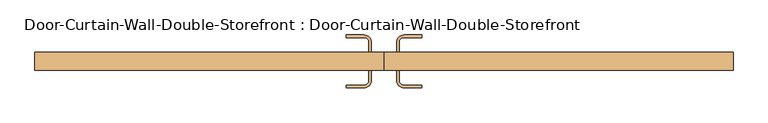
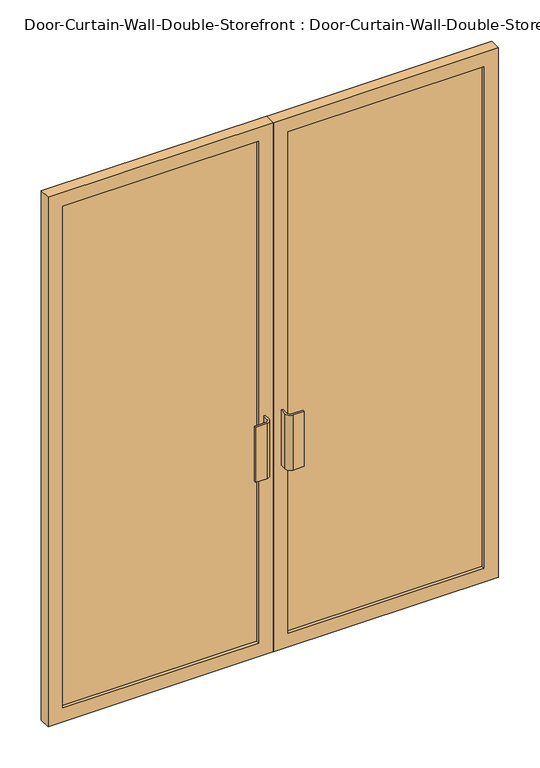
"""IFC4 building model written with IfcOpenShell, lengths in millimetres: door geometry, Door-Curtain-Wall-Double-Storefront : Door-Curtain-Wall-Double-Storefront."""

from ifc_helpers import new_model, si_unit, point, frame, frame_2d, origin, place, context, project, spatial, polyline, circle_curve, trimmed, segment, composite_curve, outline, extrude, source, transform, mapped, element, save


def door_curtain_wall_double_storefront_door_curtain_wall_double_c727979e(model_context):
    return source(origin(), model_context, "Body", "SweptSolid", [
        extrude(outline(polyline([(2190.75, 0.7668501), (0.0, 0.7668501), (0.0, 882.65), (2190.75, 882.65), (2190.75, 0.7668501)]), holes=[polyline([(2133.6, 57.9168501), (2133.6, 825.5), (57.15, 825.5), (57.15, 57.9168501), (2133.6, 57.9168501)])]), frame((0.0, 12.7, 0.0), z_axis=(0.0, 1.0, 0.0), x_axis=(0.0, 0.0, 1.0)), (0.0, 0.0, 1.0), 44.45),
        extrude(outline(polyline([(2190.75, -0.8206499), (2190.75, -882.65), (0.0, -882.65), (0.0, -0.8206499), (2190.75, -0.8206499)]), holes=[polyline([(2133.6, -825.5), (2133.6, -57.9706499), (57.15, -57.9706499), (57.15, -825.5), (2133.6, -825.5)])]), frame((0.0, 12.7, 0.0), z_axis=(0.0, 1.0, 0.0), x_axis=(0.0, 0.0, 1.0)), (0.0, 0.0, 1.0), 44.45),
        extrude(outline(polyline([(825.5, 25.4), (57.9168501, 25.4), (57.9168501, 44.45), (825.5, 44.45), (825.5, 25.4)])), frame((0.0, 0.0, 57.15), z_axis=(0.0, 0.0, 1.0), x_axis=(1.0, 0.0, 0.0)), (0.0, 0.0, 1.0), 2076.45),
        extrude(outline(polyline([(-57.9706499, 25.4), (-825.5, 25.4), (-825.5, 44.45), (-57.9706499, 44.45), (-57.9706499, 25.4)])), frame((0.0, 0.0, 57.15), z_axis=(0.0, 0.0, 1.0), x_axis=(1.0, 0.0, 0.0)), (0.0, 0.0, 1.0), 2076.45),
        extrude(outline(composite_curve([segment(polyline([(-31.7768999, 82.55), (-31.7768999, 57.15), (-38.1268999, 57.15), (-38.1268999, 82.55)]), True, "CONTINUOUS"), segment(trimmed(circle_curve(frame_2d((-50.8268999, 82.55)), 12.7), [point((-38.1268999, 82.55))], [point((-50.8268999, 95.25))], True, "CARTESIAN"), True, "CONTINUOUS"), segment(polyline([(-50.8268999, 95.25), (-95.2768999, 95.25), (-95.2768999, 101.6), (-50.8268999, 101.6)]), True, "CONTINUOUS"), segment(trimmed(circle_curve(frame_2d((-50.8268999, 82.55)), 19.05), [point((-50.8268999, 101.6))], [point((-31.7768999, 82.55))], False, "CARTESIAN"), True, "CONTINUOUS")], self_intersect=False)), frame((0.0, 0.0, 762.0), z_axis=(0.0, 0.0, 1.0), x_axis=(1.0, 0.0, 0.0)), (0.0, 0.0, 1.0), 228.6),
        extrude(outline(composite_curve([segment(trimmed(circle_curve(frame_2d((50.7731001, 82.55)), 19.05), [point((31.7231001, 82.55))], [point((50.7731001, 101.6))], False, "CARTESIAN"), True, "CONTINUOUS"), segment(polyline([(50.7731001, 101.6), (95.2231001, 101.6), (95.2231001, 95.25), (50.7731001, 95.25)]), True, "CONTINUOUS"), segment(trimmed(circle_curve(frame_2d((50.7731001, 82.55)), 12.7), [point((50.7731001, 95.25))], [point((38.0731001, 82.55))], True, "CARTESIAN"), True, "CONTINUOUS"), segment(polyline([(38.0731001, 82.55), (38.0731001, 57.15), (31.7231001, 57.15), (31.7231001, 82.55)]), True, "CONTINUOUS")], self_intersect=False)), frame((0.0, 0.0, 762.0), z_axis=(0.0, 0.0, 1.0), x_axis=(1.0, 0.0, 0.0)), (0.0, 0.0, 1.0), 228.6),
        extrude(outline(composite_curve([segment(trimmed(circle_curve(frame_2d((-50.8268999, -12.7)), 19.05), [point((-31.7768999, -12.7))], [point((-50.8268999, -31.75))], False, "CARTESIAN"), True, "CONTINUOUS"), segment(polyline([(-50.8268999, -31.75), (-95.2768999, -31.75), (-95.2768999, -25.4), (-50.8268999, -25.4)]), True, "CONTINUOUS"), segment(trimmed(circle_curve(frame_2d((-50.8268999, -12.7)), 12.7), [point((-50.8268999, -25.4))], [point((-38.1268999, -12.7))], True, "CARTESIAN"), True, "CONTINUOUS"), segment(polyline([(-38.1268999, -12.7), (-38.1268999, 12.7), (-31.7768999, 12.7), (-31.7768999, -12.7)]), True, "CONTINUOUS")], self_intersect=False)), frame((0.0, 0.0, 762.0), z_axis=(0.0, 0.0, 1.0), x_axis=(1.0, 0.0, 0.0)), (0.0, 0.0, 1.0), 228.6),
        extrude(outline(composite_curve([segment(polyline([(31.7231001, -12.7), (31.7231001, 12.7), (38.0731001, 12.7), (38.0731001, -12.7)]), True, "CONTINUOUS"), segment(trimmed(circle_curve(frame_2d((50.7731001, -12.7)), 12.7), [point((38.0731001, -12.7))], [point((50.7731001, -25.4))], True, "CARTESIAN"), True, "CONTINUOUS"), segment(polyline([(50.7731001, -25.4), (95.2231001, -25.4), (95.2231001, -31.75), (50.7731001, -31.75)]), True, "CONTINUOUS"), segment(trimmed(circle_curve(frame_2d((50.7731001, -12.7)), 19.05), [point((50.7731001, -31.75))], [point((31.7231001, -12.7))], False, "CARTESIAN"), True, "CONTINUOUS")], self_intersect=False)), frame((0.0, 0.0, 762.0), z_axis=(0.0, 0.0, 1.0), x_axis=(1.0, 0.0, 0.0)), (0.0, 0.0, 1.0), 228.6),
    ])


if __name__ == "__main__":
    model = new_model("IFC4")
    model_context = context("Model", 3, world=origin())
    ifc_project = project(units=[si_unit("LENGTHUNIT", "METRE", prefix="MILLI")], contexts=[model_context])
    site = spatial("IfcSite", under=ifc_project)
    building = spatial("IfcBuilding", under=site)
    placement = place(None, origin())
    door_curtain_wall_double_storefront_door_curtain_wall_double_shape = door_curtain_wall_double_storefront_door_curtain_wall_double_c727979e(model_context)
    element("IfcDoor", 1, ObjectType="Door-Curtain-Wall-Double-Storefront : Door-Curtain-Wall-Double-Storefront", at=placement, inside=building, context=model_context, shape_type="MappedRepresentation", body=[
        mapped(door_curtain_wall_double_storefront_door_curtain_wall_double_shape, transform((0.0, 0.0, 0.0), x_axis=(1.0, 0.0, 0.0), y_axis=(0.0, 1.0, 0.0), z_axis=(0.0, 0.0, 1.0))),
    ])
    save(model, "model.ifc")

# Revit data of these elements
# Type "Door-Curtain-Wall-Double-Storefront : Door-Curtain-Wall-Double-Storefront"
#   Type Mark = "18"
#   Construction Type Id = "opn-d46"
#   Assembly Code = "B2030100"
#   Analytic Construction = "Metal frame, double glass door"
#   Width [instance default] = 6' - 0"
#   Thermal Resistance (R) = 1.3794 (h·ft²·°F)/BTU
#   Swing Angle [instance default] = 90.00°
#   Panel Width [instance default] = 3' - 0"
#   Offset = 0' - 2 1/4"
#   Heat Transfer Coefficient (U) = 0.7250 BTU/(h·ft²·°F)
#   Define Thermal Properties by = 1
#   Function = 1
#   Frame Material = Aluminum
#   Door Handle Material = Aluminum
#   Glazing = Glass
#   Visual Light Transmittance = 0
#   Solar Heat Gain Coefficient = 0
# Element 1 (IfcDoor, "Door-Curtain-Wall-Double-Storefront : Door-Curtain-Wall-Double-Storefront")
#   Width = 5' - 9 1/2"
#   Panel Width = 2' - 10 3/4"
#   Materials on its faces: "Aluminum", "Glass"
# Materials
#   "Aluminum": class "Metal", colour RGB 247 247 247, transparency 0, Description = "Aluminum 6061", Cost = 0
#   "Glass": class "Glass", colour RGB 0 128 192, transparency 0.75, Description = "Soda Lime Glass", Cost = 0
